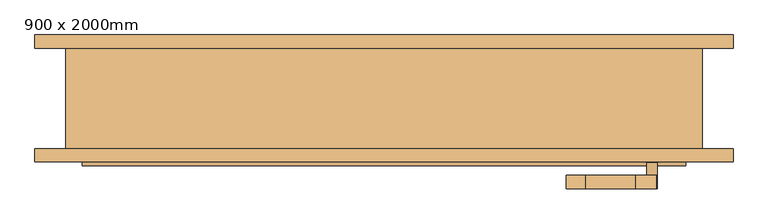
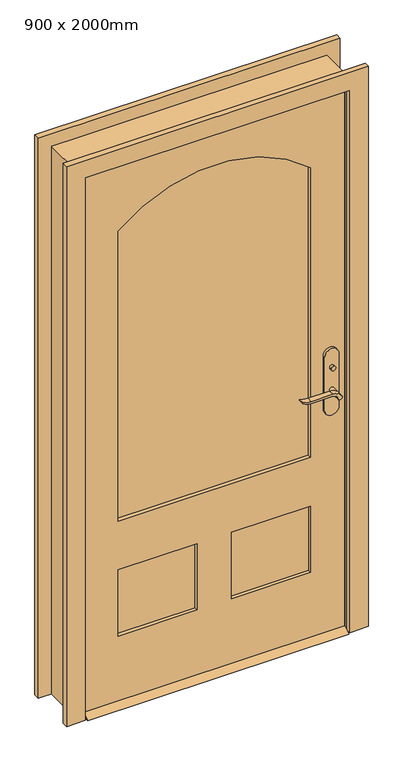
"""IFC4 building model written with IfcOpenShell, lengths in millimetres: door geometry, 900 x 2000mm."""

from ifc_helpers import new_model, si_unit, point, frame, frame_2d, origin, place, context, project, spatial, polyline, circle_curve, trimmed, segment, composite_curve, outline, extrude, faceted_brep, source, transform, mapped, element, save


def door_900_x_2000mm_520166dd(model_context):
    return source(origin(), model_context, "Body", "SolidModel", [
        extrude(outline(polyline([(-38.025, 15.0), (-12.625, 0.0), (-98.425, 0.0), (-73.025, 15.0), (-38.025, 15.0)])), frame((-457.2, 0.0, 0.0), z_axis=(1.0, 0.0, 0.0), x_axis=(0.0, 1.0, 0.0)), (0.0, 0.0, 1.0), 914.4),
        extrude(outline(polyline([(411.0, -18.025), (411.0, -28.025), (401.0, -28.025), (401.0, -18.025), (411.0, -18.025)])), frame((0.0, 0.0, 981.9), z_axis=(0.0, 0.0, 1.0), x_axis=(1.0, 0.0, 0.0)), (0.0, 0.0, 1.0), 30.0),
        extrude(outline(composite_curve([segment(trimmed(circle_curve(frame_2d((996.9, 406.0)), 8.0), [point((996.9, 398.0))], [point((996.9, 414.0))], False, "CARTESIAN"), True, "CONTINUOUS"), segment(trimmed(circle_curve(frame_2d((996.9, 406.0)), 8.0), [point((996.9, 414.0))], [point((996.9, 398.0))], False, "CARTESIAN"), True, "CONTINUOUS")], self_intersect=False)), frame((0.0, -93.025, 0.0), z_axis=(0.0, 1.0, 0.0), x_axis=(0.0, 0.0, 1.0)), (0.0, 0.0, 1.0), 10.0),
        extrude(outline(composite_curve([segment(trimmed(circle_curve(frame_2d((897.1555521, 382.3324871)), 37.2832219), [point((919.0523287, 412.5081363))], [point((934.4, 380.6325667))], False, "CARTESIAN"), True, "CONTINUOUS"), segment(polyline([(934.4, 380.6325667), (934.4, 304.3564091)]), True, "CONTINUOUS"), segment(trimmed(circle_curve(frame_2d((1017.6850638, 304.4227909)), 83.2850902), [point((934.4, 304.3564091))], [point((939.4, 276.0))], True, "CARTESIAN"), True, "CONTINUOUS"), segment(polyline([(939.4, 276.0), (936.6135558, 276.0)]), True, "CONTINUOUS"), segment(trimmed(circle_curve(frame_2d((986.6709207, 307.9396612)), 59.3791355), [point((936.6135558, 276.0))], [point((927.4, 304.3564091))], False, "CARTESIAN"), True, "CONTINUOUS"), segment(polyline([(927.4, 304.3564091), (927.4, 380.6138099)]), True, "CONTINUOUS"), segment(trimmed(circle_curve(frame_2d((909.2738613, 380.6138099)), 18.1261387), [point((927.4, 380.6138099))], [point((914.4, 398.0))], True, "CARTESIAN"), True, "CONTINUOUS"), segment(trimmed(circle_curve(frame_2d((914.4, 406.0)), 8.0), [point((914.4, 398.0))], [point((919.0523287, 412.5081363))], False, "CARTESIAN"), True, "CONTINUOUS")], self_intersect=False)), frame((0.0, 1.975, 0.0), z_axis=(0.0, 1.0, 0.0), x_axis=(0.0, 0.0, 1.0)), (0.0, 0.0, 1.0), 20.0),
        extrude(outline(composite_curve([segment(trimmed(circle_curve(frame_2d((914.4, 406.0)), 8.0), [point((914.3999903, 398.0))], [point((919.0523287, 412.5081363))], False, "CARTESIAN"), True, "CONTINUOUS"), segment(trimmed(circle_curve(frame_2d((897.1555521, 382.3324871)), 37.2832219), [point((919.0523287, 412.5081363))], [point((934.4, 380.6325667))], False, "CARTESIAN"), True, "CONTINUOUS"), segment(polyline([(934.4, 380.6325667), (934.4, 304.3564091)]), True, "CONTINUOUS"), segment(trimmed(circle_curve(frame_2d((1017.6850638, 304.4227909)), 83.2850902), [point((934.4, 304.3564091))], [point((939.4, 276.0))], True, "CARTESIAN"), True, "CONTINUOUS"), segment(polyline([(939.4, 276.0), (936.6135558, 276.0)]), True, "CONTINUOUS"), segment(trimmed(circle_curve(frame_2d((986.6709207, 307.9396612)), 59.3791355), [point((936.6135558, 276.0))], [point((927.4, 304.3564091))], False, "CARTESIAN"), True, "CONTINUOUS"), segment(polyline([(927.4, 304.3564091), (927.4, 380.6138122)]), True, "CONTINUOUS"), segment(trimmed(circle_curve(frame_2d((909.2738682, 380.6138122)), 18.1261318), [point((927.4, 380.6138122))], [point((914.3999903, 398.0))], True, "CARTESIAN"), True, "CONTINUOUS")], self_intersect=False)), frame((0.0, -133.025, 0.0), z_axis=(0.0, 1.0, 0.0), x_axis=(0.0, 0.0, 1.0)), (0.0, 0.0, 1.0), 20.0),
        extrude(outline(composite_curve([segment(trimmed(circle_curve(frame_2d((914.4, 406.0)), 8.0), [point((914.4, 398.0))], [point((914.4, 414.0))], False, "CARTESIAN"), True, "CONTINUOUS"), segment(trimmed(circle_curve(frame_2d((914.4, 406.0)), 8.0), [point((914.4, 414.0))], [point((914.4, 398.0))], False, "CARTESIAN"), True, "CONTINUOUS")], self_intersect=False)), frame((0.0, -28.025, 0.0), z_axis=(0.0, 1.0, 0.0), x_axis=(0.0, 0.0, 1.0)), (0.0, 0.0, 1.0), 30.0),
        extrude(outline(composite_curve([segment(trimmed(circle_curve(frame_2d((914.4, 406.0)), 8.0), [point((914.4, 398.0))], [point((914.4, 414.0))], False, "CARTESIAN"), True, "CONTINUOUS"), segment(trimmed(circle_curve(frame_2d((914.4, 406.0)), 8.0), [point((914.4, 414.0))], [point((914.4, 398.0))], False, "CARTESIAN"), True, "CONTINUOUS")], self_intersect=False)), frame((0.0, -113.025, 0.0), z_axis=(0.0, 1.0, 0.0), x_axis=(0.0, 0.0, 1.0)), (0.0, 0.0, 1.0), 30.0),
        extrude(outline(composite_curve([segment(polyline([(844.4, 431.0), (1039.4, 431.0)]), True, "CONTINUOUS"), segment(trimmed(circle_curve(frame_2d((1039.4, 406.0)), 25.0), [point((1039.4, 431.0))], [point((1039.4, 381.0))], False, "CARTESIAN"), True, "CONTINUOUS"), segment(polyline([(1039.4, 381.0), (844.4, 381.0)]), True, "CONTINUOUS"), segment(trimmed(circle_curve(frame_2d((844.4, 406.0)), 25.0), [point((844.4, 381.0))], [point((844.4, 431.0))], False, "CARTESIAN"), True, "CONTINUOUS")], self_intersect=False)), frame((0.0, -38.025, 0.0), z_axis=(0.0, 1.0, 0.0), x_axis=(0.0, 0.0, 1.0)), (0.0, 0.0, 1.0), 10.0),
        extrude(outline(composite_curve([segment(polyline([(844.4, 431.0), (1039.4, 431.0)]), True, "CONTINUOUS"), segment(trimmed(circle_curve(frame_2d((1039.4, 406.0)), 25.0), [point((1039.4, 431.0))], [point((1039.4, 381.0))], False, "CARTESIAN"), True, "CONTINUOUS"), segment(polyline([(1039.4, 381.0), (844.4, 381.0)]), True, "CONTINUOUS"), segment(trimmed(circle_curve(frame_2d((844.4, 406.0)), 25.0), [point((844.4, 381.0))], [point((844.4, 431.0))], False, "CARTESIAN"), True, "CONTINUOUS")], self_intersect=False)), frame((0.0, -83.025, 0.0), z_axis=(0.0, 1.0, 0.0), x_axis=(0.0, 0.0, 1.0)), (0.0, 0.0, 1.0), 10.0),
        faceted_brep([(482.2, -73.025, 0.0), (457.2, -73.025, 0.0), (457.2, -38.025, 0.0), (444.5, -38.025, 0.0), (444.5, -3.1, 0.0), (457.2, -3.1, 0.0), (457.2, 79.375, 0.0), (482.2, 79.375, 0.0), (482.2, 79.375, 2025.0), (482.2, -73.025, 2025.0), (457.2, 79.375, 2000.0), (-457.2, 79.375, 2000.0), (-457.2, 79.375, 0.0), (-482.2, 79.375, 0.0), (-482.2, 79.375, 2025.0), (457.2, -3.1, 2000.0), (444.5, -3.1, 1987.3), (-444.5, -3.1, 1987.3), (-444.5, -3.1, 0.0), (-457.2, -3.1, 0.0), (-457.2, -3.1, 2000.0), (444.5, -38.025, 1987.3), (457.2, -38.025, 2000.0), (-457.2, -38.025, 2000.0), (-457.2, -38.025, 0.0), (-444.5, -38.025, 0.0), (-444.5, -38.025, 1987.3), (457.2, -73.025, 2000.0), (-482.2, -73.025, 2025.0), (-482.2, -73.025, 0.0), (-457.2, -73.025, 0.0), (-457.2, -73.025, 2000.0)], [[[0, 1, 2, 3, 4, 5, 6, 7]], [[7, 8, 9, 0]], [[6, 10, 11, 12, 13, 14, 8, 7]], [[5, 15, 10, 6]], [[4, 16, 17, 18, 19, 20, 15, 5]], [[3, 21, 16, 4]], [[2, 22, 23, 24, 25, 26, 21, 3]], [[1, 27, 22, 2]], [[0, 9, 28, 29, 30, 31, 27, 1]], [[8, 14, 28, 9]], [[15, 20, 11, 10]], [[21, 26, 17, 16]], [[27, 31, 23, 22]], [[29, 13, 12, 19, 18, 25, 24, 30]], [[14, 13, 29, 28]], [[20, 19, 12, 11]], [[26, 25, 18, 17]], [[31, 30, 24, 23]]]),
        extrude(outline(polyline([(2000.0, -457.2), (15.0, -457.2), (15.0, 457.2), (2000.0, 457.2), (2000.0, -457.2)]), holes=[composite_curve([segment(polyline([(680.0, -337.2), (1752.35, -337.2)]), True, "CONTINUOUS"), segment(trimmed(circle_curve(frame_2d((1368.1970866, 0.0)), 511.1529134), [point((1752.35, -337.2))], [point((1752.35, 337.2))], True, "CARTESIAN"), True, "CONTINUOUS"), segment(polyline([(1752.35, 337.2), (680.0, 337.2), (680.0, -337.2)]), True, "CONTINUOUS")], self_intersect=False), polyline([(500.0, -60.325), (255.0, -60.325), (255.0, -337.2), (500.0, -337.2), (500.0, -60.325)]), polyline([(500.0, 337.2), (255.0, 337.2), (255.0, 60.325), (500.0, 60.325), (500.0, 337.2)])]), frame((0.0, -73.025, 0.0), z_axis=(0.0, 1.0, 0.0), x_axis=(0.0, 0.0, 1.0)), (0.0, 0.0, 1.0), 35.0),
        extrude(outline(composite_curve([segment(polyline([(680.0, -337.2), (680.0, 337.2), (1752.35, 337.2)]), True, "CONTINUOUS"), segment(trimmed(circle_curve(frame_2d((1368.1970866, 0.0)), 511.1529134), [point((1752.35, 337.2))], [point((1752.35, -337.2))], False, "CARTESIAN"), True, "CONTINUOUS"), segment(polyline([(1752.35, -337.2), (680.0, -337.2)]), True, "CONTINUOUS")], self_intersect=False)), frame((0.0, -59.025, 0.0), z_axis=(0.0, 1.0, 0.0), x_axis=(0.0, 0.0, 1.0)), (0.0, 0.0, 1.0), 7.0),
        extrude(outline(polyline([(-60.325, -49.6916667), (-60.325, -61.3583333), (-337.2, -61.3583333), (-337.2, -49.6916667), (-60.325, -49.6916667)])), frame((0.0, 0.0, 256.3), z_axis=(0.0, 0.0, 1.0), x_axis=(1.0, 0.0, 0.0)), (0.0, 0.0, 1.0), 243.7),
        extrude(outline(polyline([(337.2, -49.6916667), (337.2, -61.3583333), (60.325, -61.3583333), (60.325, -49.6916667), (337.2, -49.6916667)])), frame((0.0, 0.0, 255.0), z_axis=(0.0, 0.0, 1.0), x_axis=(1.0, 0.0, 0.0)), (0.0, 0.0, 1.0), 245.0),
        extrude(outline(polyline([(0.0, -463.55), (2006.35, -463.55), (2006.35, 463.55), (0.0, 463.55), (0.0, 528.55), (2071.35, 528.55), (2071.35, -528.55), (0.0, -528.55), (0.0, -463.55)])), frame((0.0, -93.025, 0.0), z_axis=(0.0, 1.0, 0.0), x_axis=(0.0, 0.0, 1.0)), (0.0, 0.0, 1.0), 20.0),
        extrude(outline(polyline([(0.0, -463.55), (2006.35, -463.55), (2006.35, 463.55), (0.0, 463.55), (0.0, 528.55), (2071.35, 528.55), (2071.35, -528.55), (0.0, -528.55), (0.0, -463.55)])), frame((0.0, 79.375, 0.0), z_axis=(0.0, 1.0, 0.0), x_axis=(0.0, 0.0, 1.0)), (0.0, 0.0, 1.0), 20.0),
    ])


if __name__ == "__main__":
    model = new_model("IFC4")
    model_context = context("Model", 3, world=origin())
    ifc_project = project(units=[si_unit("LENGTHUNIT", "METRE", prefix="MILLI")], contexts=[model_context])
    site = spatial("IfcSite", under=ifc_project)
    building = spatial("IfcBuilding", under=site)
    placement = place(None, origin())
    door_900_x_2000mm_shape = door_900_x_2000mm_520166dd(model_context)
    element("IfcDoor", 1, ObjectType="900 x 2000mm", at=placement, inside=building, context=model_context, shape_type="MappedRepresentation", body=[
        mapped(door_900_x_2000mm_shape, transform((0.0, 0.0, 0.0), x_axis=(1.0, 0.0, 0.0), y_axis=(0.0, 1.0, 0.0), z_axis=(0.0, 0.0, 1.0))),
    ])
    save(model, "model.ifc")

# Revit data of these elements
# Type "900 x 2000mm"
#   Type Mark = "9"
#   Assembly Code = "B2030100"
#   Analytic Construction = "French door, wood frame with single glass"
#   Threshold Offset [instance default] = 0' - 0.59055"
#   Thickness = 0' - 1.37795"
#   Thermal Resistance (R) = 1.0696 (h·ft²·°F)/BTU
#   Swing Angle [instance default] = 90.00°
#   Stiles = 0' - 4.72441"
#   Rough Width = 3' - 1.9685"
#   Rough Height = 6' - 7.72441"
#   Radius = 1' - 8.12413"
#   Lock Rail = 0' - 7.08661"
#   Height = 6' - 6.74016"
#   Width = 3' - 0"
#   Heat Transfer Coefficient (U) = 0.9350 BTU/(h·ft²·°F)
#   Door Offset [instance default] = 0' - 0"
#   Bottom Rail = 0' - 9.44882"
#   Threshold [instance default] = yes
#   Function = 1
#   Exterior Trim [instance default] = yes
#   Trim Material = Cherry
#   Threshold Material = Cherry
#   Panel Material = Cherry
#   Glazing = Glass
#   Frame Material = Cherry
#   Door Handle Material = Aluminum
#   Visual Light Transmittance = 0
#   Solar Heat Gain Coefficient = 0
#   Wall Closure = (empty or 0)
#   Construction Type = (empty or 0)
# Element 1 (IfcDoor, "900 x 2000mm")
#   Materials on its faces: "Cherry", "Aluminum", "Glass"
# Materials
#   "Cherry": class "Wood", colour RGB 226 177 128, transparency 0, Description = "Prunus Serotina", Cost = 0
#   "Glass": class "Glass", colour RGB 0 128 192, transparency 0.75, Description = "Soda Lime Glass", Cost = 0
#   "Aluminum": class "Metal", colour RGB 247 247 247, transparency 0, Description = "Aluminum 6061", Cost = 0
